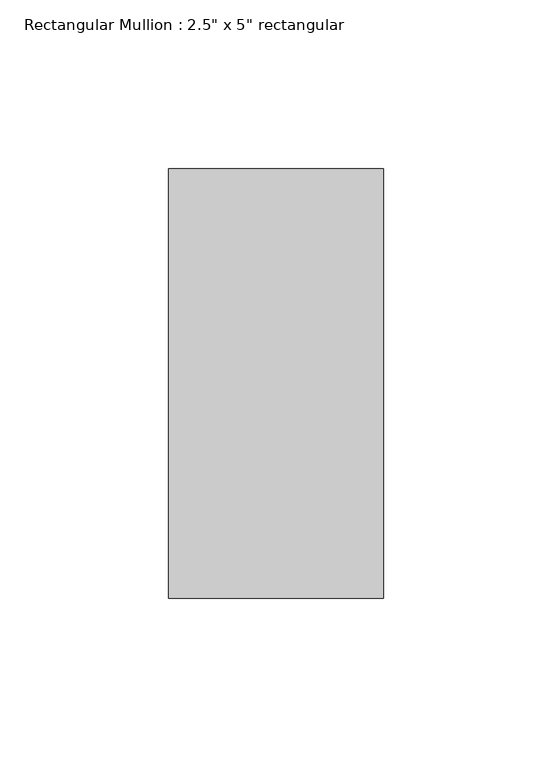
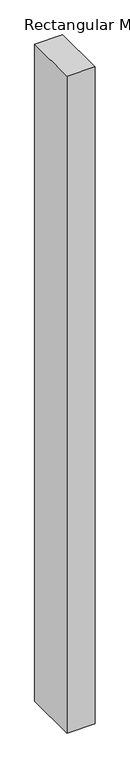
"""IFC4 building model written with IfcOpenShell, lengths in millimetres: member geometry."""

from ifc_helpers import new_model, si_unit, frame, origin, place, context, project, spatial, polyline, outline, extrude, source, transform, mapped, element, save


def member_d616553b(model_context):
    return source(origin(), model_context, "Body", "SweptSolid", [
        extrude(outline(polyline([(0.0, 63.5), (0.0, -63.5), (-63.5, -63.5), (-63.5, 63.5), (0.0, 63.5)])), frame((0.0, 0.0, -1576.4289848), z_axis=(0.0, 0.0, 1.0), x_axis=(1.0, 0.0, 0.0)), (0.0, 0.0, 1.0), 1576.4289848),
    ])


if __name__ == "__main__":
    model = new_model("IFC4")
    model_context = context("Model", 3, world=origin())
    ifc_project = project(units=[si_unit("LENGTHUNIT", "METRE", prefix="MILLI")], contexts=[model_context])
    site = spatial("IfcSite", under=ifc_project)
    building = spatial("IfcBuilding", under=site)
    placement = place(None, origin())
    member_shape = member_d616553b(model_context)
    element("IfcMember", 1, ObjectType="Rectangular Mullion : 2.5\" x 5\" rectangular", at=placement, inside=building, context=model_context, shape_type="MappedRepresentation", body=[
        mapped(member_shape, transform((0.0, 0.0, 0.0), x_axis=(1.0, 0.0, 0.0), y_axis=(0.0, 1.0, 0.0), z_axis=(0.0, 0.0, 1.0))),
    ])
    save(model, "model.ifc")

# Revit data of these elements
# Type "Rectangular Mullion : 2.5\" x 5\" rectangular"
#   built-in parameter 1007304 = 0.416667 (stored number, unit not read)
#   built-in parameter 1007301 = 0.104167 (stored number, unit not read)
#   built-in parameter 1007300 = 0.104167 (stored number, unit not read)
# Element 1 (IfcMember, "Rectangular Mullion : 2.5\" x 5\" rectangular")
#   Materials on its faces: "Aluminum"
# Materials
#   "Aluminum": class "Metal", colour RGB 247 247 247, transparency 0, Description = "Aluminum 6061", Cost = 0
